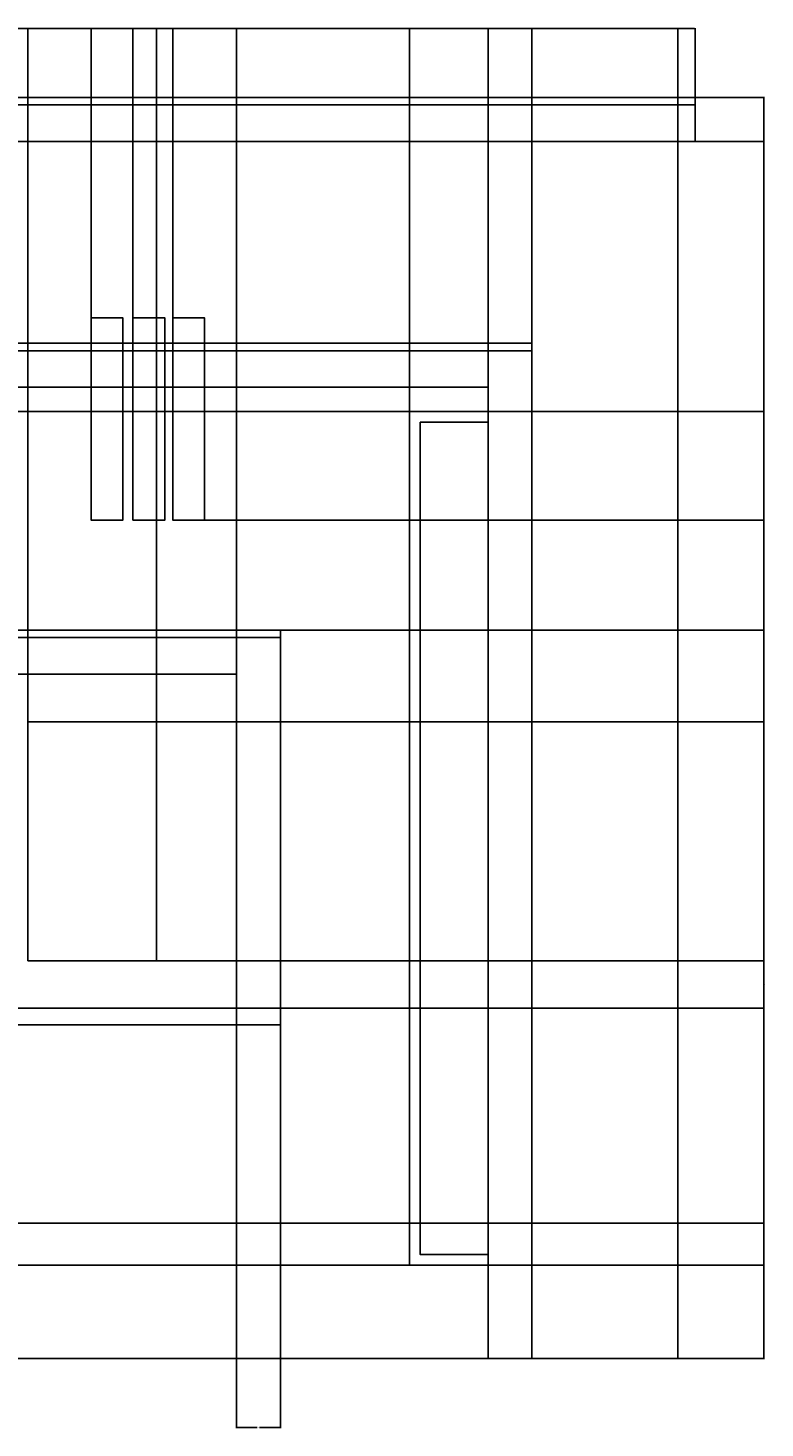
# Model space of a CAD drawing. Units: feet. Extents: x 2926 to 4178, y 965 to 1469.
# Tile 9 of 9: x 3913 to 4178, y 965 to 1469. Entities that reach past the tile are written whole.
import ezdxf

# ---------------------------------------------------------------- set-up
doc = ezdxf.new("R2010")
doc.units = ezdxf.units.FT
doc.layers.add('A-ANNO-DIMS', color=2, linetype='Continuous', lineweight=18)
doc.layers.add('A-ELEV', color=7, linetype='Continuous', lineweight=25)
doc.styles.get("Standard").update_dxf_attribs({"font": 'arial.ttf'})
doc.dimstyles.get("Standard").update_dxf_attribs({"dimtxt": 0.18, "dimasz": 0.18, "dimexe": 0.18, "dimexo": 0.0625, "dimgap": 0.09, "dimtad": 0, "dimtih": 1, "dimtoh": 1, "dimdec": 1, "dimzin": 0, "dimdsep": 46, "dimlunit": 3, "dimtxsty": 'Standard', "dimcen": 0.09, "dimadec": 0, "dimazin": 0, "dimtfac": 1, "dimtdec": 1, "dimtofl": 0, "dimtmove": 0, "dimatfit": 3, "dimfxl": 1, "dimtolj": 1, "dimtzin": 0, "dimarcsym": 0})

# ---------------------------------------------------------------- blocks, each defined once
blk = doc.blocks.new('*D74')
at = {"layer": 'A-ANNO-DIMS', "color": 0, "lineweight": -2, "transparency": 16777216}
for p, q in [((3667.11, 1298.4), (3667.11, 1468.62)), ((3667.29, 1468.44), (3909.8, 1468.44)), ((4153.1, 1468.44), (3910.59, 1468.44)), ((4153.28, 1443.71), (4153.28, 1468.62))]:
    blk.add_line(p, q, dxfattribs=at)
at = {"layer": 'A-ANNO-DIMS', "color": 0, "transparency": 16777216}
for points in [[(3667.29, 1468.47), (3667.29, 1468.41), (3667.11, 1468.44)], [(4153.1, 1468.47), (4153.1, 1468.41), (4153.28, 1468.44)]]:
    blk.add_solid(points, dxfattribs=at)
at = {"layer": 'Defpoints', "color": 0, "transparency": 16777216}
for p in [(4153.28, 1468.44), (4153.28, 1443.64), (3667.11, 1298.33)]:
    blk.add_point(p, dxfattribs=at)
at = {"layer": 'A-ANNO-DIMS', "color": 0, "transparency": 16777216, "insert": (3910.2, 1468.44), "char_height": 0.18, "attachment_point": 5}
blk.add_mtext('\\A1;486.2', dxfattribs=at)
blk = doc.blocks.new('*D75')
at = {"layer": 'A-ANNO-DIMS', "color": 0, "lineweight": -2, "transparency": 16777216}
for p, q in [((4153.34, 1443.64), (4178.26, 1443.64)), ((4178.08, 1443.46), (4178.08, 1217.17)), ((4178.08, 990.5), (4178.08, 1216.8)), ((4147.17, 990.32), (4178.26, 990.32))]:
    blk.add_line(p, q, dxfattribs=at)
at = {"layer": 'A-ANNO-DIMS', "color": 0, "transparency": 16777216}
for points in [[(4178.05, 1443.46), (4178.11, 1443.46), (4178.08, 1443.64)], [(4178.05, 990.5), (4178.11, 990.5), (4178.08, 990.32)]]:
    blk.add_solid(points, dxfattribs=at)
at = {"layer": 'Defpoints', "color": 0, "transparency": 16777216}
for p in [(4153.28, 1443.64), (4178.08, 1443.64), (4147.11, 990.32)]:
    blk.add_point(p, dxfattribs=at)
at = {"layer": 'A-ANNO-DIMS', "color": 0, "transparency": 16777216, "insert": (4178.08, 1216.98), "char_height": 0.18, "attachment_point": 5}
blk.add_mtext('\\A1;453.3', dxfattribs=at)
blk = doc.blocks.new('*D76')
at = {"layer": 'A-ANNO-DIMS', "color": 0, "lineweight": -2, "transparency": 16777216}
for p, q in [((4050.56, 1023.86), (3641.28, 1023.86)), ((3641.46, 1023.68), (3641.46, 1007.27)), ((3641.46, 990.5), (3641.46, 1006.91)), ((3667.05, 990.32), (3641.28, 990.32))]:
    blk.add_line(p, q, dxfattribs=at)
at = {"layer": 'A-ANNO-DIMS', "color": 0, "transparency": 16777216}
for points in [[(3641.43, 1023.68), (3641.49, 1023.68), (3641.46, 1023.86)], [(3641.43, 990.5), (3641.49, 990.5), (3641.46, 990.32)]]:
    blk.add_solid(points, dxfattribs=at)
at = {"layer": 'Defpoints', "color": 0, "transparency": 16777216}
for p in [(3641.46, 1023.86), (4050.62, 1023.86), (3667.11, 990.32)]:
    blk.add_point(p, dxfattribs=at)
at = {"layer": 'A-ANNO-DIMS', "color": 0, "transparency": 16777216, "insert": (3641.46, 1007.09), "char_height": 0.18, "attachment_point": 5}
blk.add_mtext('\\A1;33.53', dxfattribs=at)
blk = doc.blocks.new('*D77')
at = {"layer": 'A-ANNO-DIMS', "color": 0, "lineweight": -2, "transparency": 16777216}
for p, q in [((3782.96, 1049.98), (3641.28, 1049.98)), ((3641.46, 1049.8), (3641.46, 1037.1)), ((3641.46, 1024.04), (3641.46, 1036.74)), ((4050.56, 1023.86), (3641.28, 1023.86))]:
    blk.add_line(p, q, dxfattribs=at)
at = {"layer": 'A-ANNO-DIMS', "color": 0, "transparency": 16777216}
for points in [[(3641.43, 1049.8), (3641.49, 1049.8), (3641.46, 1049.98)], [(3641.43, 1024.04), (3641.49, 1024.04), (3641.46, 1023.86)]]:
    blk.add_solid(points, dxfattribs=at)
at = {"layer": 'Defpoints', "color": 0, "transparency": 16777216}
for p in [(3641.46, 1049.98), (3783.02, 1049.98), (4050.62, 1023.86)]:
    blk.add_point(p, dxfattribs=at)
at = {"layer": 'A-ANNO-DIMS', "color": 0, "transparency": 16777216, "insert": (3641.46, 1036.92), "char_height": 0.18, "attachment_point": 5}
blk.add_mtext('\\A1;26.13', dxfattribs=at)
blk = doc.blocks.new('*D83')
at = {"layer": 'A-ANNO-DIMS', "color": 0, "lineweight": -2, "transparency": 16777216}
for p, q in [((4050.56, 1330.74), (3641.28, 1330.74)), ((3641.46, 1330.56), (3641.46, 1314.5)), ((3641.46, 1298.08), (3641.46, 1314.14)), ((3667.05, 1297.9), (3641.28, 1297.9))]:
    blk.add_line(p, q, dxfattribs=at)
at = {"layer": 'A-ANNO-DIMS', "color": 0, "transparency": 16777216}
for points in [[(3641.43, 1330.56), (3641.49, 1330.56), (3641.46, 1330.74)], [(3641.43, 1298.08), (3641.49, 1298.08), (3641.46, 1297.9)]]:
    blk.add_solid(points, dxfattribs=at)
at = {"layer": 'Defpoints', "color": 0, "transparency": 16777216}
for p in [(3641.46, 1330.74), (4050.62, 1330.74), (3667.11, 1297.9)]:
    blk.add_point(p, dxfattribs=at)
at = {"layer": 'A-ANNO-DIMS', "color": 0, "transparency": 16777216, "insert": (3641.46, 1314.32), "char_height": 0.18, "attachment_point": 5}
blk.add_mtext('\\A1;32.85', dxfattribs=at)
blk = doc.blocks.new('*D84')
at = {"layer": 'A-ANNO-DIMS', "color": 0, "lineweight": -2, "transparency": 16777216}
for p, q in [((3757.57, 1355.28), (3641.28, 1355.28)), ((3641.46, 1355.1), (3641.46, 1343.19)), ((3641.46, 1330.92), (3641.46, 1342.83)), ((4050.56, 1330.74), (3641.28, 1330.74))]:
    blk.add_line(p, q, dxfattribs=at)
at = {"layer": 'A-ANNO-DIMS', "color": 0, "transparency": 16777216}
for points in [[(3641.43, 1355.1), (3641.49, 1355.1), (3641.46, 1355.28)], [(3641.43, 1330.92), (3641.49, 1330.92), (3641.46, 1330.74)]]:
    blk.add_solid(points, dxfattribs=at)
at = {"layer": 'Defpoints', "color": 0, "transparency": 16777216}
for p in [(3641.46, 1355.28), (3757.63, 1355.28), (4050.62, 1330.74)]:
    blk.add_point(p, dxfattribs=at)
at = {"layer": 'A-ANNO-DIMS', "color": 0, "transparency": 16777216, "insert": (3641.46, 1343.01), "char_height": 0.18, "attachment_point": 5}
blk.add_mtext('\\A1;24.533', dxfattribs=at)
blk = doc.blocks.new('*D89')
at = {"layer": 'A-ANNO-DIMS', "color": 0, "lineweight": -2, "transparency": 16777216}
for p, q in [((3913.35, 1133.35), (3913.35, 1468.62)), ((3913.53, 1468.44), (3936.04, 1468.44)), ((3959.35, 1468.44), (3936.84, 1468.44)), ((3959.53, 1133.35), (3959.53, 1468.62))]:
    blk.add_line(p, q, dxfattribs=at)
at = {"layer": 'A-ANNO-DIMS', "color": 0, "transparency": 16777216}
for points in [[(3913.53, 1468.47), (3913.53, 1468.41), (3913.35, 1468.44)], [(3959.35, 1468.47), (3959.35, 1468.41), (3959.53, 1468.44)]]:
    blk.add_solid(points, dxfattribs=at)
at = {"layer": 'Defpoints', "color": 0, "transparency": 16777216}
for p in [(3959.53, 1468.44), (3913.35, 1133.29), (3959.53, 1133.29)]:
    blk.add_point(p, dxfattribs=at)
at = {"layer": 'A-ANNO-DIMS', "color": 0, "transparency": 16777216, "insert": (3936.44, 1468.44), "char_height": 0.18, "attachment_point": 5}
blk.add_mtext('\\A1;46.18', dxfattribs=at)
blk = doc.blocks.new('*D90')
at = {"layer": 'A-ANNO-DIMS', "color": 0, "lineweight": -2, "transparency": 16777216}
for p, q in [((3959.53, 1133.35), (3959.53, 1468.62)), ((3959.71, 1468.44), (4004.77, 1468.44)), ((4050.44, 1468.44), (4005.38, 1468.44)), ((4050.62, 1023.92), (4050.62, 1468.62))]:
    blk.add_line(p, q, dxfattribs=at)
at = {"layer": 'A-ANNO-DIMS', "color": 0, "transparency": 16777216}
for points in [[(3959.71, 1468.47), (3959.71, 1468.41), (3959.53, 1468.44)], [(4050.44, 1468.47), (4050.44, 1468.41), (4050.62, 1468.44)]]:
    blk.add_solid(points, dxfattribs=at)
at = {"layer": 'Defpoints', "color": 0, "transparency": 16777216}
for p in [(4050.62, 1468.44), (3959.53, 1133.29), (4050.62, 1023.86)]:
    blk.add_point(p, dxfattribs=at)
at = {"layer": 'A-ANNO-DIMS', "color": 0, "transparency": 16777216, "insert": (4005.08, 1468.44), "char_height": 0.18, "attachment_point": 5}
blk.add_mtext('\\A1;91.1', dxfattribs=at)
blk = doc.blocks.new('*D91')
at = {"layer": 'A-ANNO-DIMS', "color": 0, "lineweight": -2, "transparency": 16777216}
for p, q in [((4050.62, 1023.92), (4050.62, 1468.62)), ((4050.8, 1468.44), (4064.4, 1468.44)), ((4078.65, 1468.44), (4065.05, 1468.44)), ((4078.83, 1023.92), (4078.83, 1468.62))]:
    blk.add_line(p, q, dxfattribs=at)
at = {"layer": 'A-ANNO-DIMS', "color": 0, "transparency": 16777216}
for points in [[(4050.8, 1468.47), (4050.8, 1468.41), (4050.62, 1468.44)], [(4078.65, 1468.47), (4078.65, 1468.41), (4078.83, 1468.44)]]:
    blk.add_solid(points, dxfattribs=at)
at = {"layer": 'Defpoints', "color": 0, "transparency": 16777216}
for p in [(4078.83, 1468.44), (4050.62, 1023.86), (4078.83, 1023.86)]:
    blk.add_point(p, dxfattribs=at)
at = {"layer": 'A-ANNO-DIMS', "color": 0, "transparency": 16777216, "insert": (4064.73, 1468.44), "char_height": 0.18, "attachment_point": 5}
blk.add_mtext('\\A1;28.2', dxfattribs=at)
blk = doc.blocks.new('*D92')
at = {"layer": 'A-ANNO-DIMS', "color": 0, "lineweight": -2, "transparency": 16777216}
for p, q in [((3959.59, 1219.22), (4178.26, 1219.22)), ((4178.08, 1219.04), (4178.08, 1176.44)), ((4178.08, 1133.47), (4178.08, 1176.07)), ((3959.59, 1133.29), (4178.26, 1133.29))]:
    blk.add_line(p, q, dxfattribs=at)
at = {"layer": 'A-ANNO-DIMS', "color": 0, "transparency": 16777216}
for points in [[(4178.05, 1219.04), (4178.11, 1219.04), (4178.08, 1219.22)], [(4178.05, 1133.47), (4178.11, 1133.47), (4178.08, 1133.29)]]:
    blk.add_solid(points, dxfattribs=at)
at = {"layer": 'Defpoints', "color": 0, "transparency": 16777216}
for p in [(3959.53, 1219.22), (4178.08, 1219.22), (3959.53, 1133.29)]:
    blk.add_point(p, dxfattribs=at)
at = {"layer": 'A-ANNO-DIMS', "color": 0, "transparency": 16777216, "insert": (4178.08, 1176.25), "char_height": 0.18, "attachment_point": 5}
blk.add_mtext('\\A1;85.93', dxfattribs=at)
blk = doc.blocks.new('*D97')
at = {"layer": 'A-ANNO-DIMS', "color": 0, "lineweight": -2, "transparency": 16777216}
for p, q in [((3888.93, 1355.34), (3888.93, 1468.62)), ((3889.11, 1468.44), (3912.1, 1468.44)), ((3935.88, 1468.44), (3912.89, 1468.44)), ((3936.06, 1364.46), (3936.06, 1468.62))]:
    blk.add_line(p, q, dxfattribs=at)
at = {"layer": 'A-ANNO-DIMS', "color": 0, "transparency": 16777216}
for points in [[(3889.11, 1468.47), (3889.11, 1468.41), (3888.93, 1468.44)], [(3935.88, 1468.47), (3935.88, 1468.41), (3936.06, 1468.44)]]:
    blk.add_solid(points, dxfattribs=at)
at = {"layer": 'Defpoints', "color": 0, "transparency": 16777216}
for p in [(3936.06, 1468.44), (3936.06, 1364.4), (3888.93, 1355.28)]:
    blk.add_point(p, dxfattribs=at)
at = {"layer": 'A-ANNO-DIMS', "color": 0, "transparency": 16777216, "insert": (3912.49, 1468.44), "char_height": 0.18, "attachment_point": 5}
blk.add_mtext('\\A1;47.13', dxfattribs=at)
blk = doc.blocks.new('*D98')
at = {"layer": 'A-ANNO-DIMS', "color": 0, "lineweight": -2, "transparency": 16777216}
for p, q in [((3936.06, 1364.46), (3936.06, 1468.62)), ((3936.24, 1468.44), (3943.2, 1468.44)), ((3950.94, 1468.44), (3943.98, 1468.44)), ((3951.12, 1364.46), (3951.12, 1468.62))]:
    blk.add_line(p, q, dxfattribs=at)
at = {"layer": 'A-ANNO-DIMS', "color": 0, "transparency": 16777216}
for points in [[(3936.24, 1468.47), (3936.24, 1468.41), (3936.06, 1468.44)], [(3950.94, 1468.47), (3950.94, 1468.41), (3951.12, 1468.44)]]:
    blk.add_solid(points, dxfattribs=at)
at = {"layer": 'Defpoints', "color": 0, "transparency": 16777216}
for p in [(3951.12, 1468.44), (3936.06, 1364.4), (3951.12, 1364.4)]:
    blk.add_point(p, dxfattribs=at)
at = {"layer": 'A-ANNO-DIMS', "color": 0, "transparency": 16777216, "insert": (3943.59, 1468.44), "char_height": 0.18, "attachment_point": 5}
blk.add_mtext('\\A1;15.06', dxfattribs=at)
blk = doc.blocks.new('*D99')
at = {"layer": 'A-ANNO-DIMS', "color": 0, "lineweight": -2, "transparency": 16777216}
for p, q in [((3951.12, 1364.46), (3951.12, 1468.62)), ((3951.3, 1468.44), (3957.81, 1468.44)), ((3965.24, 1468.44), (3958.72, 1468.44)), ((3965.42, 1364.46), (3965.42, 1468.62))]:
    blk.add_line(p, q, dxfattribs=at)
at = {"layer": 'A-ANNO-DIMS', "color": 0, "transparency": 16777216}
for points in [[(3951.3, 1468.47), (3951.3, 1468.41), (3951.12, 1468.44)], [(3965.24, 1468.47), (3965.24, 1468.41), (3965.42, 1468.44)]]:
    blk.add_solid(points, dxfattribs=at)
at = {"layer": 'Defpoints', "color": 0, "transparency": 16777216}
for p in [(3965.42, 1468.44), (3951.12, 1364.4), (3965.42, 1364.4)]:
    blk.add_point(p, dxfattribs=at)
at = {"layer": 'A-ANNO-DIMS', "color": 0, "transparency": 16777216, "insert": (3958.27, 1468.44), "char_height": 0.18, "attachment_point": 5}
blk.add_mtext('\\A1;14.298', dxfattribs=at)
blk = doc.blocks.new('*D100')
at = {"layer": 'A-ANNO-DIMS', "color": 0, "lineweight": -2, "transparency": 16777216}
for p, q in [((3965.42, 1364.46), (3965.42, 1468.62)), ((3965.6, 1468.44), (4021.74, 1468.44)), ((4078.65, 1468.44), (4022.51, 1468.44)), ((4078.83, 1339.53), (4078.83, 1468.62))]:
    blk.add_line(p, q, dxfattribs=at)
at = {"layer": 'A-ANNO-DIMS', "color": 0, "transparency": 16777216}
for points in [[(3965.6, 1468.47), (3965.6, 1468.41), (3965.42, 1468.44)], [(4078.65, 1468.47), (4078.65, 1468.41), (4078.83, 1468.44)]]:
    blk.add_solid(points, dxfattribs=at)
at = {"layer": 'Defpoints', "color": 0, "transparency": 16777216}
for p in [(4078.83, 1468.44), (3965.42, 1364.4), (4078.83, 1339.46)]:
    blk.add_point(p, dxfattribs=at)
at = {"layer": 'A-ANNO-DIMS', "color": 0, "transparency": 16777216, "insert": (4022.12, 1468.44), "char_height": 0.18, "attachment_point": 5}
blk.add_mtext('\\A1;113.4', dxfattribs=at)
blk = doc.blocks.new('*D101')
at = {"layer": 'A-ANNO-DIMS', "color": 0, "lineweight": -2, "transparency": 16777216}
for p, q in [((4078.83, 1339.53), (4078.83, 1468.62)), ((4079.01, 1468.44), (4086.28, 1468.44)), ((4094.46, 1468.44), (4087.19, 1468.44)), ((4094.64, 1355.34), (4094.64, 1468.62))]:
    blk.add_line(p, q, dxfattribs=at)
at = {"layer": 'A-ANNO-DIMS', "color": 0, "transparency": 16777216}
for points in [[(4079.01, 1468.47), (4079.01, 1468.41), (4078.83, 1468.44)], [(4094.46, 1468.47), (4094.46, 1468.41), (4094.64, 1468.44)]]:
    blk.add_solid(points, dxfattribs=at)
at = {"layer": 'Defpoints', "color": 0, "transparency": 16777216}
for p in [(4094.64, 1468.44), (4094.64, 1355.28), (4078.83, 1339.46)]:
    blk.add_point(p, dxfattribs=at)
at = {"layer": 'A-ANNO-DIMS', "color": 0, "transparency": 16777216, "insert": (4086.73, 1468.44), "char_height": 0.18, "attachment_point": 5}
blk.add_mtext('\\A1;15.814', dxfattribs=at)
blk = doc.blocks.new('*D102')
at = {"layer": 'A-ANNO-DIMS', "color": 0, "lineweight": -2, "transparency": 16777216}
for p, q in [((4094.64, 1355.34), (4094.64, 1468.62)), ((4094.82, 1468.44), (4120.48, 1468.44)), ((4146.93, 1468.44), (4121.27, 1468.44)), ((4147.11, 1427.89), (4147.11, 1468.62))]:
    blk.add_line(p, q, dxfattribs=at)
at = {"layer": 'A-ANNO-DIMS', "color": 0, "transparency": 16777216}
for points in [[(4094.82, 1468.47), (4094.82, 1468.41), (4094.64, 1468.44)], [(4146.93, 1468.47), (4146.93, 1468.41), (4147.11, 1468.44)]]:
    blk.add_solid(points, dxfattribs=at)
at = {"layer": 'Defpoints', "color": 0, "transparency": 16777216}
for p in [(4147.11, 1468.44), (4147.11, 1427.83), (4094.64, 1355.28)]:
    blk.add_point(p, dxfattribs=at)
at = {"layer": 'A-ANNO-DIMS', "color": 0, "transparency": 16777216, "insert": (4120.88, 1468.44), "char_height": 0.18, "attachment_point": 5}
blk.add_mtext('\\A1;52.47', dxfattribs=at)
blk = doc.blocks.new('*D103')
at = {"layer": 'A-ANNO-DIMS', "color": 0, "lineweight": -2, "transparency": 16777216}
for p, q in [((4147.11, 1427.89), (4147.11, 1468.62)), ((4147.29, 1468.44), (4149.8, 1468.44)), ((4153.1, 1468.44), (4150.59, 1468.44)), ((4153.28, 1443.71), (4153.28, 1468.62))]:
    blk.add_line(p, q, dxfattribs=at)
at = {"layer": 'A-ANNO-DIMS', "color": 0, "transparency": 16777216}
for points in [[(4147.29, 1468.47), (4147.29, 1468.41), (4147.11, 1468.44)], [(4153.1, 1468.47), (4153.1, 1468.41), (4153.28, 1468.44)]]:
    blk.add_solid(points, dxfattribs=at)
at = {"layer": 'Defpoints', "color": 0, "transparency": 16777216}
for p in [(4153.28, 1468.44), (4153.28, 1443.64), (4147.11, 1427.83)]:
    blk.add_point(p, dxfattribs=at)
at = {"layer": 'A-ANNO-DIMS', "color": 0, "transparency": 16777216, "insert": (4150.2, 1468.44), "char_height": 0.18, "attachment_point": 5}
blk.add_mtext('\\A1;6.169', dxfattribs=at)
blk = doc.blocks.new('*D104')
at = {"layer": 'A-ANNO-DIMS', "color": 0, "lineweight": -2, "transparency": 16777216}
for p, q in [((4153.34, 1443.64), (4178.26, 1443.64)), ((4178.08, 1443.46), (4178.08, 1435.92)), ((4178.08, 1428.01), (4178.08, 1435.56)), ((4153.34, 1427.83), (4178.26, 1427.83))]:
    blk.add_line(p, q, dxfattribs=at)
at = {"layer": 'A-ANNO-DIMS', "color": 0, "transparency": 16777216}
for points in [[(4178.05, 1443.46), (4178.11, 1443.46), (4178.08, 1443.64)], [(4178.05, 1428.01), (4178.11, 1428.01), (4178.08, 1427.83)]]:
    blk.add_solid(points, dxfattribs=at)
at = {"layer": 'Defpoints', "color": 0, "transparency": 16777216}
for p in [(4153.28, 1443.64), (4178.08, 1443.64), (4153.28, 1427.83)]:
    blk.add_point(p, dxfattribs=at)
at = {"layer": 'A-ANNO-DIMS', "color": 0, "transparency": 16777216, "insert": (4178.08, 1435.74), "char_height": 0.18, "attachment_point": 5}
blk.add_mtext('\\A1;15.814', dxfattribs=at)
blk = doc.blocks.new('*D107')
at = {"layer": 'A-ANNO-DIMS', "color": 0, "lineweight": -2, "transparency": 16777216}
for p, q in [((3976.94, 1291.73), (4178.26, 1291.73)), ((4178.08, 1291.55), (4178.08, 1272.12)), ((4178.08, 1252.32), (4178.08, 1271.75)), ((4004.19, 1252.14), (4178.26, 1252.14))]:
    blk.add_line(p, q, dxfattribs=at)
at = {"layer": 'A-ANNO-DIMS', "color": 0, "transparency": 16777216}
for points in [[(4178.05, 1291.55), (4178.11, 1291.55), (4178.08, 1291.73)], [(4178.05, 1252.32), (4178.11, 1252.32), (4178.08, 1252.14)]]:
    blk.add_solid(points, dxfattribs=at)
at = {"layer": 'Defpoints', "color": 0, "transparency": 16777216}
for p in [(3976.87, 1291.73), (4178.08, 1291.73), (4004.12, 1252.14)]:
    blk.add_point(p, dxfattribs=at)
at = {"layer": 'A-ANNO-DIMS', "color": 0, "transparency": 16777216, "insert": (4178.08, 1271.94), "char_height": 0.18, "attachment_point": 5}
blk.add_mtext('\\A1;39.596', dxfattribs=at)
blk = doc.blocks.new('*D108')
at = {"layer": 'A-ANNO-DIMS', "color": 0, "lineweight": -2, "transparency": 16777216}
for p, q in [((4078.89, 1330.74), (4178.26, 1330.74)), ((4178.08, 1330.56), (4178.08, 1177.48)), ((4178.08, 1024.04), (4178.08, 1177.12)), ((4078.89, 1023.86), (4178.26, 1023.86))]:
    blk.add_line(p, q, dxfattribs=at)
at = {"layer": 'A-ANNO-DIMS', "color": 0, "transparency": 16777216}
for points in [[(4178.05, 1330.56), (4178.11, 1330.56), (4178.08, 1330.74)], [(4178.05, 1024.04), (4178.11, 1024.04), (4178.08, 1023.86)]]:
    blk.add_solid(points, dxfattribs=at)
at = {"layer": 'Defpoints', "color": 0, "transparency": 16777216}
for p in [(4078.83, 1330.74), (4178.08, 1330.74), (4078.83, 1023.86)]:
    blk.add_point(p, dxfattribs=at)
at = {"layer": 'A-ANNO-DIMS', "color": 0, "transparency": 16777216, "insert": (4178.08, 1177.3), "char_height": 0.18, "attachment_point": 5}
blk.add_mtext('\\A1;306.9', dxfattribs=at)
blk = doc.blocks.new('*D126')
at = {"layer": 'A-ANNO-DIMS', "color": 0, "lineweight": -2, "transparency": 16777216}
for p, q in [((3988.31, 1116.26), (3988.31, 965.34)), ((4004.12, 1110.26), (4004.12, 965.34)), ((3988.49, 965.52), (3995.76, 965.52)), ((4003.94, 965.52), (3996.67, 965.52))]:
    blk.add_line(p, q, dxfattribs=at)
at = {"layer": 'A-ANNO-DIMS', "color": 0, "transparency": 16777216}
for points in [[(3988.49, 965.55), (3988.49, 965.49), (3988.31, 965.52)], [(4003.94, 965.55), (4003.94, 965.49), (4004.12, 965.52)]]:
    blk.add_solid(points, dxfattribs=at)
at = {"layer": 'Defpoints', "color": 0, "transparency": 16777216}
for p in [(3988.31, 1116.32), (4004.12, 1110.32), (4004.12, 965.52)]:
    blk.add_point(p, dxfattribs=at)
at = {"layer": 'A-ANNO-DIMS', "color": 0, "transparency": 16777216, "insert": (3996.22, 965.52), "char_height": 0.18, "attachment_point": 5}
blk.add_mtext('\\A1;15.814', dxfattribs=at)
blk = doc.blocks.new('*D127')
at = {"layer": 'A-ANNO-DIMS', "color": 0, "lineweight": -2, "transparency": 16777216}
for p, q in [((3959.53, 1219.28), (3959.53, 1468.62)), ((3959.71, 1468.44), (3973.52, 1468.44)), ((3988.13, 1468.44), (3974.31, 1468.44)), ((3988.31, 1236.39), (3988.31, 1468.62))]:
    blk.add_line(p, q, dxfattribs=at)
at = {"layer": 'A-ANNO-DIMS', "color": 0, "transparency": 16777216}
for points in [[(3959.71, 1468.47), (3959.71, 1468.41), (3959.53, 1468.44)], [(3988.13, 1468.47), (3988.13, 1468.41), (3988.31, 1468.44)]]:
    blk.add_solid(points, dxfattribs=at)
at = {"layer": 'Defpoints', "color": 0, "transparency": 16777216}
for p in [(3988.31, 1468.44), (3988.31, 1236.32), (3959.53, 1219.22)]:
    blk.add_point(p, dxfattribs=at)
at = {"layer": 'A-ANNO-DIMS', "color": 0, "transparency": 16777216, "insert": (3973.92, 1468.44), "char_height": 0.18, "attachment_point": 5}
blk.add_mtext('\\A1;28.78', dxfattribs=at)
blk = doc.blocks.new('*D128')
at = {"layer": 'A-ANNO-DIMS', "color": 0, "lineweight": -2, "transparency": 16777216}
for p, q in [((3959.59, 1133.29), (4178.26, 1133.29)), ((4178.08, 1133.11), (4178.08, 1124.99)), ((4178.08, 1116.5), (4178.08, 1124.62)), ((3988.37, 1116.32), (4178.26, 1116.32))]:
    blk.add_line(p, q, dxfattribs=at)
at = {"layer": 'A-ANNO-DIMS', "color": 0, "transparency": 16777216}
for points in [[(4178.05, 1133.11), (4178.11, 1133.11), (4178.08, 1133.29)], [(4178.05, 1116.5), (4178.11, 1116.5), (4178.08, 1116.32)]]:
    blk.add_solid(points, dxfattribs=at)
at = {"layer": 'Defpoints', "color": 0, "transparency": 16777216}
for p in [(3959.53, 1133.29), (4178.08, 1133.29), (3988.31, 1116.32)]:
    blk.add_point(p, dxfattribs=at)
at = {"layer": 'A-ANNO-DIMS', "color": 0, "transparency": 16777216, "insert": (4178.08, 1124.81), "char_height": 0.18, "attachment_point": 5}
blk.add_mtext('\\A1;16.963', dxfattribs=at)
blk = doc.blocks.new('*D129')
at = {"layer": 'A-ANNO-DIMS', "color": 0, "lineweight": -2, "transparency": 16777216}
for p, q in [((4004.19, 1038.92), (4178.26, 1038.92)), ((4178.08, 1038.74), (4178.08, 1014.8)), ((4178.08, 990.5), (4178.08, 1014.44)), ((4078.89, 990.32), (4178.26, 990.32))]:
    blk.add_line(p, q, dxfattribs=at)
at = {"layer": 'A-ANNO-DIMS', "color": 0, "transparency": 16777216}
for points in [[(4178.05, 1038.74), (4178.11, 1038.74), (4178.08, 1038.92)], [(4178.05, 990.5), (4178.11, 990.5), (4178.08, 990.32)]]:
    blk.add_solid(points, dxfattribs=at)
at = {"layer": 'Defpoints', "color": 0, "transparency": 16777216}
for p in [(4004.12, 1038.92), (4078.83, 990.32), (4178.08, 990.32)]:
    blk.add_point(p, dxfattribs=at)
at = {"layer": 'A-ANNO-DIMS', "color": 0, "transparency": 16777216, "insert": (4178.08, 1014.62), "char_height": 0.18, "attachment_point": 5}
blk.add_mtext('\\A1;48.6', dxfattribs=at)

msp = doc.modelspace()

# ---------------------------------------------------------------- linework, layer by layer
at = {"layer": 'A-ELEV'}
for p, q in [((3868.4052, 1440.9727), (4153.2808, 1440.9727)), ((4153.2808, 1427.8302), (4153.2808, 1443.6445)), ((4147.1119, 990.3246), (4147.1119, 1427.8302)), ((3757.63, 1352.606), (4094.6412, 1352.606)), ((4078.8269, 1339.4635), (4078.8269, 990.3246)), ((3667.1119, 1249.4671), (4004.1232, 1249.4671)), ((4004.1232, 1110.3246), (4004.1232, 1252.1389)), ((3667.1119, 1236.3246), (3988.3089, 1236.3246)), ((3988.3089, 1110.3246), (3988.3089, 1236.3246)), ((3888.9271, 1116.3246), (3988.3089, 1116.3246)), ((3667.1119, 1110.3246), (4004.1232, 1110.3246)), ((4004.1232, 1110.3246), (4004.1232, 1038.9216)), ((4004.1232, 1038.9216), (3888.9271, 1038.9216)), ((3667.1119, 990.3246), (4147.1119, 990.3246))]:
    msp.add_line(p, q, dxfattribs=at)
for points in [[(4153.2808, 1443.6445), (3868.4052, 1443.6445), (3868.4052, 1427.8302), (4153.2808, 1427.8302)], [(4094.6412, 990.3246), (4094.6412, 1355.2778), (3757.63, 1355.2778), (3757.63, 1339.4635), (4078.8269, 1339.4635)], [(4078.8269, 1326.907), (4054.4618, 1326.907), (4054.4618, 1027.6935), (4078.8269, 1027.6935)], [(4004.1232, 1236.3246), (4004.1232, 1252.1389), (3667.1119, 1252.1389), (3667.1119, 1236.3246), (3988.3089, 1236.3246)]]:
    msp.add_lwpolyline(points, dxfattribs=at)
for points in [[(3936.0598, 1364.3965), (3947.5164, 1364.3965), (3947.5164, 1291.7348), (3936.0598, 1291.7348)], [(3951.1199, 1364.3965), (3962.5765, 1364.3965), (3962.5765, 1291.7348), (3951.1199, 1291.7348)], [(3965.4182, 1364.3965), (3976.8747, 1364.3965), (3976.8747, 1291.7348), (3965.4182, 1291.7348)], [(4078.8269, 1330.7444), (4050.6244, 1330.7444), (4050.6244, 1023.8561), (4078.8269, 1023.8561)], [(3913.3516, 1219.2195), (3959.5291, 1219.2195), (3959.5291, 1133.2879), (3913.3516, 1133.2879)]]:
    msp.add_lwpolyline(points, close=True, dxfattribs=at)

# ---------------------------------------------------------------- dimensions: what is measured, and where the dimension line sits
at = {"layer": 'A-ANNO-DIMS'}
for base, p1, p2, override, picture, middle in [((4153.2808, 1468.4445), (3667.1119, 1298.3338), (4153.2808, 1443.6445), {"dimdec": 1, "dimlfac": 1, "dimrnd": 0, "dimzin": 0, "dimdsep": 46, "dimlunit": 2}, '*D74', (3910.1964, 1468.4445)), ((3936.0598, 1468.4445), (3888.9271, 1355.2778), (3936.0598, 1364.3965), {"dimdec": 2, "dimlfac": 1, "dimrnd": 0, "dimzin": 0, "dimdsep": 46, "dimlunit": 2}, '*D97', (3912.4935, 1468.4445)), ((3959.5291, 1468.4445), (3913.3516, 1133.2879), (3959.5291, 1133.2879), {"dimdec": 2, "dimlfac": 1, "dimrnd": 0, "dimzin": 0, "dimdsep": 46, "dimlunit": 2}, '*D89', (3936.4404, 1468.4445)), ((3951.1199, 1468.4445), (3936.0598, 1364.3965), (3951.1199, 1364.3965), {"dimdec": 2, "dimlfac": 1, "dimrnd": 0, "dimzin": 0, "dimdsep": 46, "dimlunit": 2}, '*D98', (3943.5899, 1468.4445)), ((3965.4182, 1468.4445), (3951.1199, 1364.3965), (3965.4182, 1364.3965), {"dimdec": 3, "dimlfac": 1, "dimrnd": 0, "dimzin": 0, "dimdsep": 46, "dimlunit": 2}, '*D99', (3958.269, 1468.4445)), ((4050.6244, 1468.4445), (3959.5291, 1133.2879), (4050.6244, 1023.8561), {"dimdec": 1, "dimlfac": 1, "dimrnd": 0, "dimzin": 0, "dimdsep": 46, "dimlunit": 2}, '*D90', (4005.0768, 1468.4445)), ((3988.3089, 1468.4445), (3959.5291, 1219.2195), (3988.3089, 1236.3246), {"dimdec": 2, "dimlfac": 1, "dimrnd": 0, "dimzin": 0, "dimdsep": 46, "dimlunit": 2}, '*D127', (3973.919, 1468.4445)), ((4078.8269, 1468.4445), (3965.4182, 1364.3965), (4078.8269, 1339.4635), {"dimdec": 1, "dimlfac": 1, "dimrnd": 0, "dimzin": 0, "dimdsep": 46, "dimlunit": 2}, '*D100', (4022.1226, 1468.4445)), ((4078.8269, 1468.4445), (4050.6244, 1023.8561), (4078.8269, 1023.8561), {"dimdec": 1, "dimlfac": 1, "dimrnd": 0, "dimzin": 0, "dimdsep": 46, "dimlunit": 2}, '*D91', (4064.7257, 1468.4445)), ((4094.6412, 1468.4445), (4078.8269, 1339.4635), (4094.6412, 1355.2778), {"dimdec": 3, "dimlfac": 1, "dimrnd": 0, "dimzin": 0, "dimdsep": 46, "dimlunit": 2}, '*D101', (4086.7341, 1468.4445)), ((4147.1119, 1468.4445), (4094.6412, 1355.2778), (4147.1119, 1427.8302), {"dimdec": 2, "dimlfac": 1, "dimrnd": 0, "dimzin": 0, "dimdsep": 46, "dimlunit": 2}, '*D102', (4120.8766, 1468.4445)), ((4153.2808, 1468.4445), (4147.1119, 1427.8302), (4153.2808, 1443.6445), {"dimdec": 3, "dimlfac": 1, "dimrnd": 0, "dimzin": 0, "dimdsep": 46, "dimlunit": 2}, '*D103', (4150.1964, 1468.4445)), ((4004.1232, 965.5246), (3988.3089, 1116.3246), (4004.1232, 1110.3246), {"dimdec": 3, "dimlfac": 1, "dimrnd": 0, "dimzin": 0, "dimdsep": 46, "dimlunit": 2}, '*D126', (3996.216, 965.5246))]:
    dim = msp.add_linear_dim(base=base, p1=p1, p2=p2, dimstyle='Standard', override=override, dxfattribs=at)
    dim.commit()
    dim.dimension.update_dxf_attribs({"geometry": picture, "text_midpoint": middle})
for base, p1, p2, override, picture, middle in [((4178.0808, 1443.6445), (4147.1119, 990.3246), (4153.2808, 1443.6445), {"dimdec": 1, "dimlfac": 1, "dimrnd": 0, "dimzin": 0, "dimdsep": 46, "dimlunit": 2}, '*D75', (4178.0808, 1216.9845)), ((4178.0808, 1443.6445), (4153.2808, 1427.8302), (4153.2808, 1443.6445), {"dimdec": 3, "dimlfac": 1, "dimrnd": 0, "dimzin": 0, "dimdsep": 46, "dimlunit": 2}, '*D104', (4178.0808, 1435.7374)), ((3641.4599, 1355.2778), (4050.6244, 1330.7444), (3757.63, 1355.2778), {"dimdec": 3, "dimlfac": 1, "dimrnd": 0, "dimzin": 0, "dimdsep": 46, "dimlunit": 2}, '*D84', (3641.4599, 1343.0111)), ((3641.4599, 1330.7444), (3667.1119, 1297.8963), (4050.6244, 1330.7444), {"dimdec": 2, "dimlfac": 1, "dimrnd": 0, "dimzin": 0, "dimdsep": 46, "dimlunit": 2}, '*D83', (3641.4599, 1314.3203)), ((4178.0808, 1330.7444), (4078.8269, 1023.8561), (4078.8269, 1330.7444), {"dimdec": 1, "dimlfac": 1, "dimrnd": 0, "dimzin": 0, "dimdsep": 46, "dimlunit": 2}, '*D108', (4178.0808, 1177.3002)), ((4178.0808, 1291.7348), (4004.1232, 1252.1389), (3976.8747, 1291.7348), {"dimdec": 3, "dimlfac": 1, "dimrnd": 0, "dimzin": 0, "dimdsep": 46, "dimlunit": 2}, '*D107', (4178.0808, 1271.9368)), ((4178.0808, 1219.2195), (3959.5291, 1133.2879), (3959.5291, 1219.2195), {"dimdec": 2, "dimlfac": 1, "dimrnd": 0, "dimzin": 0, "dimdsep": 46, "dimlunit": 2}, '*D92', (4178.0808, 1176.2537)), ((4178.0808, 1133.2879), (3988.3089, 1116.3246), (3959.5291, 1133.2879), {"dimdec": 3, "dimlfac": 1, "dimrnd": 0, "dimzin": 0, "dimdsep": 46, "dimlunit": 2}, '*D128', (4178.0808, 1124.8062)), ((3641.4599, 1049.9841), (4050.6244, 1023.8561), (3783.0229, 1049.9841), {"dimdec": 2, "dimlfac": 1, "dimrnd": 0, "dimzin": 0, "dimdsep": 46, "dimlunit": 2}, '*D77', (3641.4599, 1036.9201)), ((4178.0808, 990.3246), (4004.1232, 1038.9216), (4078.8269, 990.3246), {"dimdec": 1, "dimlfac": 1, "dimrnd": 0, "dimzin": 0, "dimdsep": 46, "dimlunit": 2}, '*D129', (4178.0808, 1014.6231)), ((3641.4599, 1023.8561), (3667.1119, 990.3246), (4050.6244, 1023.8561), {"dimdec": 2, "dimlfac": 1, "dimrnd": 0, "dimzin": 0, "dimdsep": 46, "dimlunit": 2}, '*D76', (3641.4599, 1007.0903))]:
    dim = msp.add_linear_dim(base=base, p1=p1, p2=p2, angle=90, dimstyle='Standard', override=override, dxfattribs=at)
    dim.commit()
    dim.dimension.update_dxf_attribs({"geometry": picture, "text_midpoint": middle})

doc.saveas('drawing.dxf')
